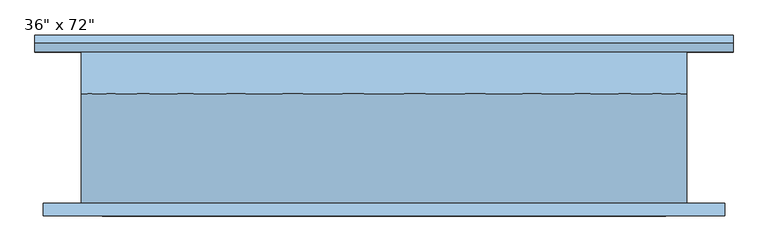
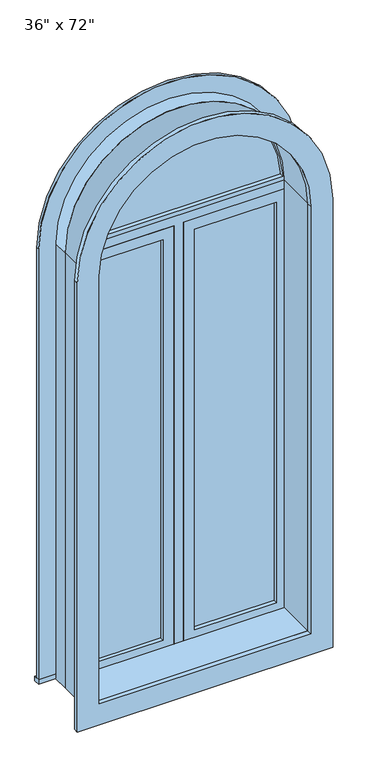
"""IFC4 building model written with IfcOpenShell, lengths in millimetres: window geometry."""

from ifc_helpers import new_model, si_unit, point, frame, frame_2d, origin, place, context, project, spatial, polyline, circle_curve, trimmed, segment, composite_curve, outline, extrude, source, transform, mapped, element, save


def window_e7489165(model_context):
    return source(origin(), model_context, "Body", "SweptSolid", [
        extrude(outline(composite_curve([segment(polyline([(2152.65, -506.3478419), (247.65, -506.3478419), (247.65, 522.3521581), (2152.65, 522.3521581)]), True, "CONTINUOUS"), segment(trimmed(circle_curve(frame_2d((2152.65, 8.0021581)), 514.35), [point((2152.65, 522.3521581))], [point((2152.65, -506.3478419))], False, "CARTESIAN"), True, "CONTINUOUS")], self_intersect=False), holes=[composite_curve([segment(trimmed(circle_curve(frame_2d((2152.65, 8.0021581)), 425.45), [point((2152.65, -417.4478419))], [point((2152.65, 433.4521581))], True, "CARTESIAN"), True, "CONTINUOUS"), segment(polyline([(2152.65, 433.4521581), (336.55, 433.4521581), (336.55, -417.4478419), (2152.65, -417.4478419)]), True, "CONTINUOUS")], self_intersect=False)]), frame((0.0, -133.35, 0.0), z_axis=(0.0, 1.0, 0.0), x_axis=(0.0, 0.0, 1.0)), (0.0, 0.0, 1.0), 19.05),
        extrude(outline(composite_curve([segment(trimmed(circle_curve(frame_2d((2152.65, 8.0021581)), 419.2154707), [point((2171.6999995, 426.7845699))], [point((2171.6999995, -410.7802537))], False, "CARTESIAN"), True, "CONTINUOUS"), segment(polyline([(2171.6999995, -410.7802537), (2171.6999995, 426.7845699)]), True, "CONTINUOUS")], self_intersect=False)), frame((0.0, 66.675, 0.0), z_axis=(0.0, 1.0, 0.0), x_axis=(0.0, 0.0, 1.0)), (0.0, 0.0, 1.0), 12.7),
        extrude(outline(composite_curve([segment(trimmed(circle_curve(frame_2d((2152.65, 8.0021581)), 438.15), [point((2152.65, 446.1521581))], [point((2152.65, -430.1478419))], False, "CARTESIAN"), True, "CONTINUOUS"), segment(polyline([(2152.65, -430.1478419), (2152.65, 446.1521581)]), True, "CONTINUOUS")], self_intersect=False), holes=[composite_curve([segment(polyline([(2171.6999995, 426.7845698), (2171.6999995, -410.7802537)]), True, "CONTINUOUS"), segment(trimmed(circle_curve(frame_2d((2152.65, 8.0021581)), 419.2154707), [point((2171.6999995, -410.7802537))], [point((2171.6999995, 426.7845698))], True, "CARTESIAN"), True, "CONTINUOUS")], self_intersect=False)]), frame((0.0, 50.8, 0.0), z_axis=(0.0, 1.0, 0.0), x_axis=(0.0, 0.0, 1.0)), (0.0, 0.0, 1.0), 44.45),
        extrude(outline(composite_curve([segment(polyline([(304.8, -449.1978419), (304.8, 465.2021581), (2152.65, 465.2021581)]), True, "CONTINUOUS"), segment(trimmed(circle_curve(frame_2d((2152.65, 8.0021581)), 457.2), [point((2152.65, 465.2021581))], [point((2152.65, -449.1978419))], False, "CARTESIAN"), True, "CONTINUOUS"), segment(polyline([(2152.65, -449.1978419), (304.8, -449.1978419)]), True, "CONTINUOUS")], self_intersect=False), holes=[composite_curve([segment(polyline([(323.85, -430.1478419), (2152.65, -430.1478419)]), True, "CONTINUOUS"), segment(trimmed(circle_curve(frame_2d((2152.65, 8.0021581)), 438.15), [point((2152.65, -430.1478419))], [point((2152.65, 446.1521581))], True, "CARTESIAN"), True, "CONTINUOUS"), segment(polyline([(2152.65, 446.1521581), (323.85, 446.1521581), (323.85, -430.1478419)]), True, "CONTINUOUS")], self_intersect=False)]), frame((0.0, 50.8, 0.0), z_axis=(0.0, 1.0, 0.0), x_axis=(0.0, 0.0, 1.0)), (0.0, 0.0, 1.0), 63.5),
        extrude(outline(polyline([(71.5021581, 79.375), (401.7021581, 79.375), (401.7021581, 66.675), (71.5021581, 66.675), (71.5021581, 79.375)])), frame((0.0, 0.0, 368.3), z_axis=(0.0, 0.0, 1.0), x_axis=(1.0, 0.0, 0.0)), (0.0, 0.0, 1.0), 1701.8),
        extrude(outline(polyline([(2114.55, 27.0521581), (323.85, 27.0521581), (323.85, 446.1521581), (2114.55, 446.1521581), (2114.55, 27.0521581)]), holes=[polyline([(2070.1, 71.5021581), (2070.1, 401.7021581), (368.3, 401.7021581), (368.3, 71.5021581), (2070.1, 71.5021581)])]), frame((0.0, 50.8, 0.0), z_axis=(0.0, 1.0, 0.0), x_axis=(0.0, 0.0, 1.0)), (0.0, 0.0, 1.0), 44.45),
        extrude(outline(polyline([(323.85, -11.0478419), (323.85, 27.0521581), (2114.55, 27.0521581), (2114.55, 446.1521581), (2152.65, 446.1521581), (2152.65, -430.1478419), (2114.55, -430.1478419), (2114.55, -11.0478419), (323.85, -11.0478419)])), frame((0.0, 50.8, 0.0), z_axis=(0.0, 1.0, 0.0), x_axis=(0.0, 0.0, 1.0)), (0.0, 0.0, 1.0), 63.5),
        extrude(outline(polyline([(-519.0478419, 139.7), (535.0521581, 139.7), (535.0521581, 114.3), (-519.0478419, 114.3), (-519.0478419, 139.7)])), frame((0.0, 0.0, 304.8), z_axis=(0.0, 0.0, 1.0), x_axis=(1.0, 0.0, 0.0)), (0.0, 0.0, 1.0), 19.05),
        extrude(outline(composite_curve([segment(polyline([(323.85, 446.1521581), (323.85, 535.0521581), (2152.65, 535.0521581)]), True, "CONTINUOUS"), segment(trimmed(circle_curve(frame_2d((2152.65, 8.0021581)), 527.05), [point((2152.65, 535.0521581))], [point((2152.65, -519.0478419))], False, "CARTESIAN"), True, "CONTINUOUS"), segment(polyline([(2152.65, -519.0478419), (323.85, -519.0478419), (323.85, -430.1478419), (2152.65, -430.1478419)]), True, "CONTINUOUS"), segment(trimmed(circle_curve(frame_2d((2152.65, 8.0021581)), 438.15), [point((2152.65, -430.1478419))], [point((2152.65, 446.1521581))], True, "CARTESIAN"), True, "CONTINUOUS"), segment(polyline([(2152.65, 446.1521581), (323.85, 446.1521581)]), True, "CONTINUOUS")], self_intersect=False)), frame((0.0, 114.3, 0.0), z_axis=(0.0, 1.0, 0.0), x_axis=(0.0, 0.0, 1.0)), (0.0, 0.0, 1.0), 12.7),
        extrude(outline(polyline([(-55.4978419, 66.675), (-385.6978419, 66.675), (-385.6978419, 79.375), (-55.4978419, 79.375), (-55.4978419, 66.675)])), frame((0.0, 0.0, 368.3), z_axis=(0.0, 0.0, 1.0), x_axis=(1.0, 0.0, 0.0)), (0.0, 0.0, 1.0), 1701.8),
        extrude(outline(polyline([(2114.55, -430.1478419), (323.85, -430.1478419), (323.85, -11.0478419), (2114.55, -11.0478419), (2114.55, -430.1478419)]), holes=[polyline([(2070.1, -385.6978419), (2070.1, -55.4978419), (368.3, -55.4978419), (368.3, -385.6978419), (2070.1, -385.6978419)])]), frame((0.0, 50.8, 0.0), z_axis=(0.0, 1.0, 0.0), x_axis=(0.0, 0.0, 1.0)), (0.0, 0.0, 1.0), 44.45),
        extrude(outline(composite_curve([segment(polyline([(304.8, 465.2021581), (2152.65, 465.2021581)]), True, "CONTINUOUS"), segment(trimmed(circle_curve(frame_2d((2152.65, 8.0021581)), 457.2), [point((2152.65, 465.2021581))], [point((2152.65, -449.1978419))], False, "CARTESIAN"), True, "CONTINUOUS"), segment(polyline([(2152.65, -449.1978419), (304.8, -449.1978419), (304.8, 465.2021581)]), True, "CONTINUOUS")], self_intersect=False), holes=[composite_curve([segment(polyline([(336.55, 433.4521581), (336.55, -417.4478419), (2152.65, -417.4478419)]), True, "CONTINUOUS"), segment(trimmed(circle_curve(frame_2d((2152.65, 8.0021581)), 425.45), [point((2152.65, -417.4478419))], [point((2152.65, 433.4521581))], True, "CARTESIAN"), True, "CONTINUOUS"), segment(polyline([(2152.65, 433.4521581), (336.55, 433.4521581)]), True, "CONTINUOUS")], self_intersect=False)]), frame((0.0, -114.3, 0.0), z_axis=(0.0, 1.0, 0.0), x_axis=(0.0, 0.0, 1.0)), (0.0, 0.0, 1.0), 165.1),
    ])


if __name__ == "__main__":
    model = new_model("IFC4")
    model_context = context("Model", 3, world=origin())
    ifc_project = project(units=[si_unit("LENGTHUNIT", "METRE", prefix="MILLI")], contexts=[model_context])
    site = spatial("IfcSite", under=ifc_project)
    building = spatial("IfcBuilding", under=site)
    placement = place(None, origin())
    window_shape = window_e7489165(model_context)
    element("IfcWindow", 1, ObjectType="36\" x 72\"", at=placement, inside=building, context=model_context, shape_type="MappedRepresentation", body=[
        mapped(window_shape, transform((0.0, 0.0, 0.0), x_axis=(1.0, 0.0, 0.0), y_axis=(0.0, 1.0, 0.0), z_axis=(0.0, 0.0, 1.0))),
    ])
    save(model, "model.ifc")

# Revit data of these elements
# Type "36\" x 72\""
#   Type Mark = "10"
#   Construction Type Id = "SGL"
#   Assembly Code = "B2020100"
#   Analytic Construction = "Large single-glazed windows"
#   Visual Light Transmittance = 0.9
#   Solar Heat Gain Coefficient = 0.86
#   Heat Transfer Coefficient (U) = 0.979472 BTU/(h·ft²·°F)
#   Height = 6' - 0"
#   Default Sill Height = 1' - 0"
#   Trim Projection - Ext. = 0' - 0 1/2"
#   Trim Projection - Int. = 0' - 0 3/4"
#   Trim Width - Exterior = 0' - 3 1/2"
#   Trim Width - Interior = 0' - 3 1/2"
#   Width = 3' - 0"
#   Window Inset = 0' - 0 3/4"
#   Define Thermal Properties by = 1
#   Glass Pane Material = Glass
#   Sash Material = Sash
#   Trim Exterior Material = Trim
#   Trim Interior Material = Trim
#   Wall Closure = (empty or 0)
# Element 1 (IfcWindow, "36\" x 72\"")
#   Materials on its faces: "Sash", "Trim", "Glass"
# Materials
#   "Glass": class "Glass", colour RGB 0 128 192, transparency 0.75, Description = "Soda Lime Glass", Cost = 0
#   "Sash": class "Wood", colour RGB 224 178 126, transparency 0
#   "Trim": class "Wood", colour RGB 224 178 126, transparency 0
